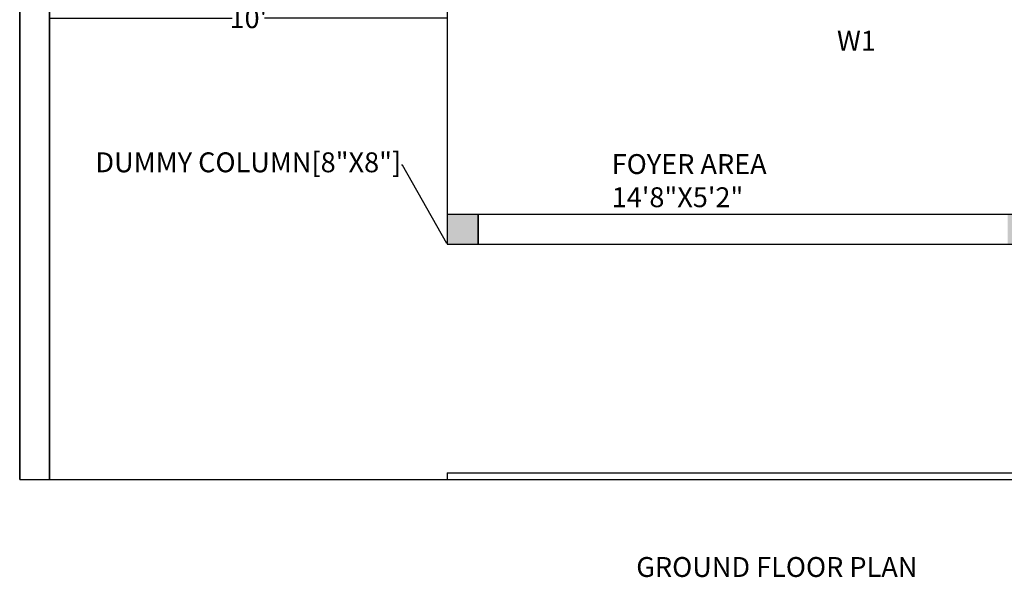
# Model space of a CAD drawing. Units: inches. Extents: x -36302355 to 648, y -221479757 to 75.
# Tile 2 of 37: x 145 to 442, y -752 to -583. Entities that reach past the tile are written whole.
import ezdxf
from ezdxf import colors
from ezdxf.entities.mleader import LeaderData, LeaderLine
from ezdxf.math import Vec2, Vec3

# ---------------------------------------------------------------- set-up
doc = ezdxf.new("R2010")
doc.units = ezdxf.units.IN
doc.header["$MEASUREMENT"] = 0
for name, color, linetype, lineweight in [('A-ANNO-DIMS', 2, 'Continuous', 18), ('A-ANNO-IDEN', 7, 'Continuous', 18), ('A-ANNO-TEXT', 7, 'Continuous', 18), ('A-ANNO-TITL', 7, 'Continuous', 25), ('A-AREA-IDEN', 7, 'Continuous', 18), ('A-COLS', 7, 'Continuous', 35), ('A-COLS-PATT', 242, 'Continuous', 13), ('A-FLOR', 8, 'Continuous', 25), ('A-WALL', 7, 'Continuous', 35), ('L-WALL', 7, 'Continuous', 30)]:
    doc.layers.add(name, color=color, linetype=linetype, lineweight=lineweight)
doc.styles.get("Standard").update_dxf_attribs({"font": 'arial.ttf'})
doc.dimstyles.get("Standard").update_dxf_attribs({"dimtxt": 0.18, "dimasz": 0.18, "dimexe": 0.18, "dimexo": 0.0625, "dimgap": 0.09, "dimtad": 0, "dimtih": 1, "dimtoh": 1, "dimdec": 0, "dimzin": 0, "dimdsep": 46, "dimlunit": 3, "dimtxsty": 'Standard', "dimcen": 0.09, "dimadec": 0, "dimazin": 0, "dimtfac": 1, "dimtdec": 0, "dimtofl": 0, "dimtmove": 0, "dimatfit": 3, "dimfxl": 1, "dimtolj": 1, "dimtzin": 0, "dimarcsym": 0})

# ---------------------------------------------------------------- blocks, each defined once
blk = doc.blocks.new('*D6')
at = {"layer": 'A-ANNO-DIMS', "color": 0, "lineweight": -2, "transparency": 16777216}
for p, q in [((154.2, -580.08), (154.2, -583.08)), ((274.2, -580.08), (274.2, -583.08)), ((154.38, -582.9), (209.3, -582.9)), ((274.02, -582.9), (219.1, -582.9))]:
    blk.add_line(p, q, dxfattribs=at)
at = {"layer": 'A-ANNO-DIMS', "color": 0, "transparency": 16777216}
for points in [[(154.38, -582.87), (154.38, -582.93), (154.2, -582.9)], [(274.02, -582.87), (274.02, -582.93), (274.2, -582.9)]]:
    blk.add_solid(points, dxfattribs=at)
at = {"layer": 'Defpoints', "color": 0, "transparency": 16777216}
for p in [(154.2, -580.02), (274.2, -580.02), (274.2, -582.9)]:
    blk.add_point(p, dxfattribs=at)
at = {"layer": 'A-ANNO-DIMS', "color": 0, "transparency": 16777216, "insert": (214.2, -582.9), "char_height": 6, "attachment_point": 5}
blk.add_mtext("\\A1;10'", dxfattribs=at)

msp = doc.modelspace()

# ---------------------------------------------------------------- hatches: boundary and pattern name
at = {"layer": 'A-COLS-PATT'}
h = msp.add_hatch(color=256, dxfattribs=at)
h.dxf.hatch_style = 1
h.paths.add_polyline_path([(283.54, -642.02), (274.2, -642.02), (274.2, -651.02), (283.54, -651.02)])
h.paths.add_polyline_path([(452.2, -642.02), (443.43, -642.02), (443.43, -651.02), (452.2, -651.02)])

# ---------------------------------------------------------------- linework, layer by layer
at = {"layer": 'A-COLS'}
msp.add_line((283.54, -642.02), (283.54, -651.02), dxfattribs=at)
at = {"layer": 'A-FLOR'}
for p, q in [((274.2, -580.02), (274.2, -651.02)), ((274.2, -642.02), (605.2, -642.02)), ((274.2, -651.02), (605.2, -651.02))]:
    msp.add_line(p, q, dxfattribs=at)
at = {"layer": 'A-WALL'}
for p, q in [((145.2, -167.02), (145.2, -722.02)), ((154.2, -167.02), (154.2, -722.02))]:
    msp.add_line(p, q, dxfattribs=at)
at = {"layer": 'L-WALL'}
for p, q in [((145.2, -722.02), (605.2, -722.02)), ((274.2, -720.02), (274.2, -720.02)), ((274.2, -720.02), (274.2, -722.02)), ((274.2, -720.02), (605.2, -720.02))]:
    msp.add_line(p, q, dxfattribs=at)

# ---------------------------------------------------------------- texts
at = {"layer": 'A-ANNO-IDEN', "insert": (391.89, -586.7), "char_height": 6, "attachment_point": 1}
msp.add_mtext_dynamic_manual_height_columns('W1', width=0.8021, gutter_width=1, heights=[0], dxfattribs=at)
at = {"layer": 'A-ANNO-TITL', "insert": (331.3, -745.45), "char_height": 6, "attachment_point": 1}
msp.add_mtext('GROUND FLOOR PLAN', dxfattribs=at)
at = {"layer": 'A-AREA-IDEN', "insert": (323.9, -623.91), "char_height": 6, "attachment_point": 1}
msp.add_mtext('FOYER AREA\\P14\'8"X5\'2"', dxfattribs=at)

# ---------------------------------------------------------------- dimensions: what is measured, and where the dimension line sits
at = {"layer": 'A-ANNO-DIMS'}
dim = msp.add_linear_dim(base=(274.2, -582.9), p1=(154.2, -580.02), p2=(274.2, -580.02), dimstyle='Standard', override={"dimtxt": 6, "dimclrd": 0, "dimclre": 0, "dimclrt": 0}, dxfattribs=at)
dim.commit()
dim.dimension.update_dxf_attribs({"geometry": '*D6', "text_midpoint": (214.2, -582.9)})

# ---------------------------------------------------------------- leaders
at = {"layer": 'A-ANNO-TEXT'}
ml = msp.add_multileader_mtext('Standard', dxfattribs=at)
ml.set_content('DUMMY COLUMN[8"X8"]', color=256)
ml.set_leader_properties()
ml.build(insert=Vec2(0, 0))
ml.multileader.update_dxf_attribs({"dogleg_length": 0.36, "arrow_head_size": 0.18})
ctx = ml.context
ctx.base_point, ctx.char_height, ctx.arrow_head_size, ctx.landing_gap_size, ctx.plane_origin = Vec3(165.6, -627.22), 6, 0.18, 0.09, Vec3(274.2, -651.02)
ctx.text_align_type = 2
notes = []
notes.append((ctx, [(0, (1, 1, 0), (260.79, -627.22), (-1, 0), 0.36, [(0, [(274.2, -651.02)], 0, [])])]))
ctx.mtext.insert, ctx.mtext.alignment, ctx.mtext.flow_direction = Vec3(260.34, -623.38), 3, 5
for ctx, leaders in notes:
    for number, flags, end, landing, length, lines in leaders:
        leader = LeaderData()
        leader.index, (leader.has_last_leader_line, leader.has_dogleg_vector, leader.attachment_direction) = number, flags
        leader.last_leader_point, leader.dogleg_vector, leader.dogleg_length = Vec3(end), Vec3(landing), length
        for number, points, colour, breaks in lines:
            line = LeaderLine()
            line.index, line.vertices, line.color, line.breaks = number, Vec3.list(points), colors.encode_raw_color(colour), breaks
            leader.lines.append(line)
        ctx.leaders.append(leader)

doc.saveas('drawing.dxf')
